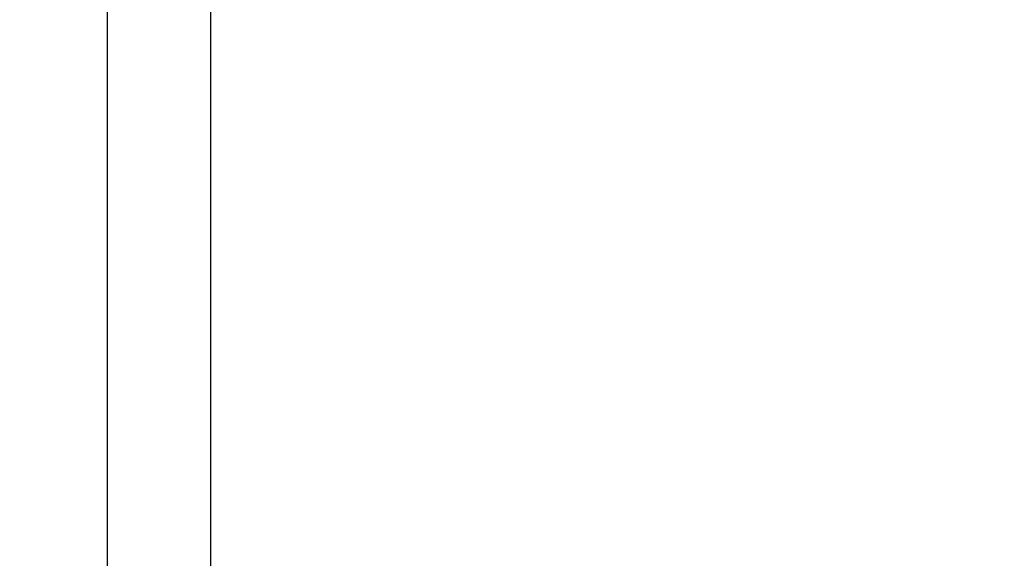
# Model space of a CAD drawing. Units: millimetres. Extents: x 595116 to 630915, y 909473 to 920225.
# Tile 52 of 134: x 629500 to 629559, y 919314 to 919346. Entities that reach past the tile are written whole.
import ezdxf

# ---------------------------------------------------------------- set-up
doc = ezdxf.new("R2010")
doc.units = ezdxf.units.MM
doc.layers.add('Dimension', color=3, linetype='Continuous', lineweight=18)
doc.styles.get("Standard").update_dxf_attribs({"font": 'arial.ttf'})
doc.dimstyles.new('ISO-25', dxfattribs={"dimtxt": 9, "dimasz": 6, "dimexe": 1.25, "dimexo": 0.625, "dimtad": 1, "dimlunit": 4, "dimtxsty": 'Standard', "dimcen": 2.5, "dimadec": 0, "dimazin": 0, "dimtfac": 1, "dimtmove": 0, "dimatfit": 3, "dimfxl": 1, "dimarcsym": 0})

# ---------------------------------------------------------------- blocks, each defined once
blk = doc.blocks.new('*D215')
at = {"layer": 'Defpoints', "color": 0, "transparency": 16777216}
for p in [(629316.041, 919411.828), (629505.041, 919411.828), (629505.041, 918832.378)]:
    blk.add_point(p, dxfattribs=at)
at = {"layer": 'Dimension', "color": 0, "lineweight": -2, "transparency": 16777216}
for p, q in [((629316.041, 919411.203), (629316.041, 918831.128)), ((629505.041, 919411.203), (629505.041, 918831.128)), ((629322.041, 918832.378), (629499.041, 918832.378))]:
    blk.add_line(p, q, dxfattribs=at)
at = {"layer": 'Dimension', "color": 0, "transparency": 16777216}
for points in [[(629322.041, 918833.378), (629322.041, 918831.378), (629316.041, 918832.378)], [(629499.041, 918833.378), (629499.041, 918831.378), (629505.041, 918832.378)]]:
    blk.add_solid(points, dxfattribs=at)
at = {"layer": 'Dimension', "color": 0, "transparency": 16777216, "insert": (629410.541, 918837.598), "char_height": 9, "attachment_point": 5}
blk.add_mtext('15\'-9"', dxfattribs=at)
blk = doc.blocks.new('*D216')
at = {"layer": 'Defpoints', "color": 0, "transparency": 16777216}
for p in [(629505.041, 919411.828), (629743.541, 919411.928), (629743.541, 918832.378)]:
    blk.add_point(p, dxfattribs=at)
at = {"layer": 'Dimension', "color": 0, "lineweight": -2, "transparency": 16777216}
for p, q in [((629505.041, 919411.203), (629505.041, 918831.128)), ((629743.541, 919411.303), (629743.541, 918831.128)), ((629511.041, 918832.378), (629737.541, 918832.378))]:
    blk.add_line(p, q, dxfattribs=at)
at = {"layer": 'Dimension', "color": 0, "transparency": 16777216}
for points in [[(629511.041, 918833.378), (629511.041, 918831.378), (629505.041, 918832.378)], [(629737.541, 918833.378), (629737.541, 918831.378), (629743.541, 918832.378)]]:
    blk.add_solid(points, dxfattribs=at)
at = {"layer": 'Dimension', "color": 0, "transparency": 16777216, "insert": (629624.291, 918837.656), "char_height": 9, "attachment_point": 5}
blk.add_mtext('19\'-10 1/2"', dxfattribs=at)
blk = doc.blocks.new('*D220')
at = {"layer": 'Defpoints', "color": 0, "transparency": 16777216}
for p in [(629824.951, 920160.756), (629511.274, 919302.009), (629824.951, 919302.009)]:
    blk.add_point(p, dxfattribs=at)
at = {"layer": 'Dimension', "color": 0, "lineweight": -2, "transparency": 16777216}
for p, q in [((629511.274, 919302.634), (629511.274, 920162.006)), ((629824.951, 919302.634), (629824.951, 920162.006)), ((629517.274, 920160.756), (629818.951, 920160.756))]:
    blk.add_line(p, q, dxfattribs=at)
at = {"layer": 'Dimension', "color": 0, "transparency": 16777216}
for points in [[(629517.274, 920161.756), (629517.274, 920159.756), (629511.274, 920160.756)], [(629818.951, 920161.756), (629818.951, 920159.756), (629824.951, 920160.756)]]:
    blk.add_solid(points, dxfattribs=at)
at = {"layer": 'Dimension', "color": 0, "transparency": 16777216, "insert": (629668.113, 920166.035), "char_height": 9, "attachment_point": 5}
blk.add_mtext('26\'-1 1/2"', dxfattribs=at)

msp = doc.modelspace()

# ---------------------------------------------------------------- dimensions: what is measured, and where the dimension line sits
at = {"layer": 'Dimension'}
for base, p1, p2, picture, middle in [((629824.951, 920160.756), (629511.274, 919302.009), (629824.951, 919302.009), '*D220', (629668.113, 920166.035)), ((629505.041, 918832.378), (629316.041, 919411.828), (629505.041, 919411.828), '*D215', (629410.541, 918837.598)), ((629743.541, 918832.378), (629505.041, 919411.828), (629743.541, 919411.928), '*D216', (629624.291, 918837.656))]:
    dim = msp.add_linear_dim(base=base, p1=p1, p2=p2, dimstyle='ISO-25', override={"dimdec": 1, "dimlfac": 1, "dimrnd": 0, "dimzin": 1, "dimdsep": 46, "dimlunit": 4, "dimfrac": 2}, dxfattribs=at)
    dim.commit()
    dim.dimension.update_dxf_attribs({"geometry": picture, "text_midpoint": middle})

doc.saveas('drawing.dxf')
